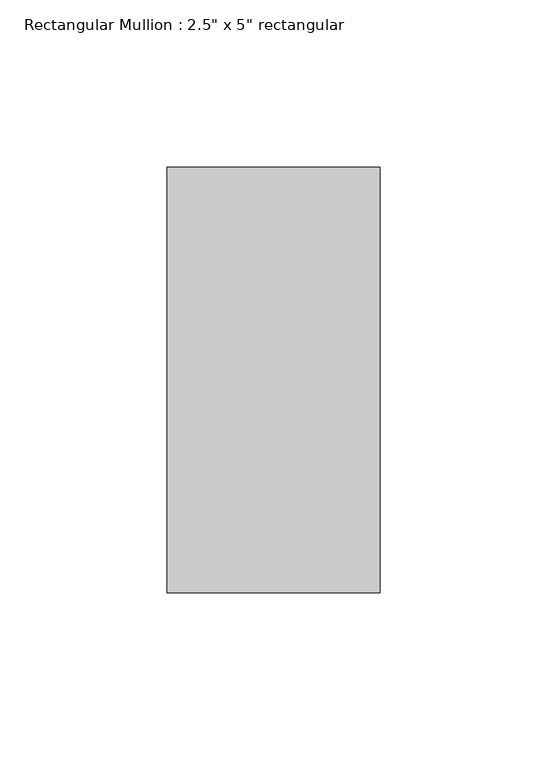
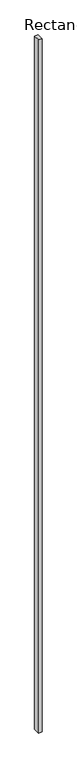
"""IFC4 building model written with IfcOpenShell, lengths in millimetres: member geometry."""

from ifc_helpers import new_model, si_unit, frame, origin, place, context, project, spatial, polyline, outline, extrude, source, transform, mapped, element, save


def member_6474a55f(model_context):
    return source(origin(), model_context, "Body", "SweptSolid", [
        extrude(outline(polyline([(0.0, 63.5), (0.0, -63.5), (-63.5, -63.5), (-63.5, 63.5), (0.0, 63.5)])), frame((0.0, 0.0, -13659.3142857), z_axis=(0.0, 0.0, 1.0), x_axis=(1.0, 0.0, 0.0)), (0.0, 0.0, 1.0), 13659.3142857),
    ])


if __name__ == "__main__":
    model = new_model("IFC4")
    model_context = context("Model", 3, world=origin())
    ifc_project = project(units=[si_unit("LENGTHUNIT", "METRE", prefix="MILLI")], contexts=[model_context])
    site = spatial("IfcSite", under=ifc_project)
    building = spatial("IfcBuilding", under=site)
    placement = place(None, origin())
    member_shape = member_6474a55f(model_context)
    element("IfcMember", 1, ObjectType="Rectangular Mullion : 2.5\" x 5\" rectangular", at=placement, inside=building, context=model_context, shape_type="MappedRepresentation", body=[
        mapped(member_shape, transform((0.0, 0.0, 0.0), x_axis=(1.0, 0.0, 0.0), y_axis=(0.0, 1.0, 0.0), z_axis=(0.0, 0.0, 1.0))),
    ])
    save(model, "model.ifc")

# Revit data of these elements
# Type "Rectangular Mullion : 2.5\" x 5\" rectangular"
#   built-in parameter 1007304 = 0.416667 (stored number, unit not read)
#   built-in parameter 1007301 = 0.104167 (stored number, unit not read)
#   built-in parameter 1007300 = 0.104167 (stored number, unit not read)
# Element 1 (IfcMember, "Rectangular Mullion : 2.5\" x 5\" rectangular")
#   Materials on its faces: "Aluminum"
# Materials
#   "Aluminum": class "Metal", colour RGB 247 247 247, transparency 0, Description = "Aluminum 6061", Cost = 0
